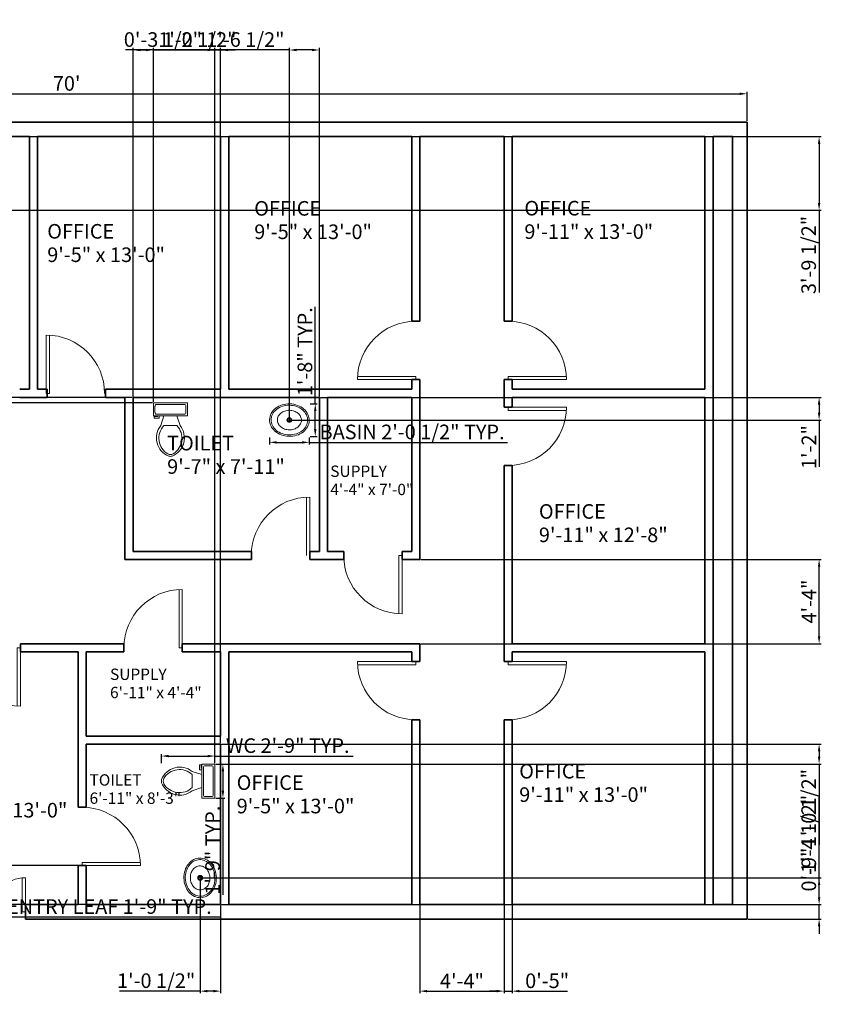
# Model space of a CAD drawing. Units: inches. Extents: x 2070 to 3026, y 1437 to 2044.
# Tile 2 of 2: x 2524 to 3026, y 1437 to 2044. Entities that reach past the tile are written whole.
import ezdxf

# ---------------------------------------------------------------- set-up
doc = ezdxf.new("R2010")
doc.units = ezdxf.units.IN
doc.layers.add('A-ANNO-DIMS', color=11, linetype='Continuous', lineweight=18, true_color=0xf27172)
for name, color, linetype, lineweight in [('A-AREA-IDEN', 7, 'Continuous', 18), ('A-DOOR', 4, 'Continuous', 18), ('A-FLOR-FIXT', 8, 'Continuous', 18), ('A-WALL', 7, 'Continuous', 35)]:
    doc.layers.add(name, color=color, linetype=linetype, lineweight=lineweight)
doc.styles.get("Standard").update_dxf_attribs({"font": 'arial.ttf'})
doc.dimstyles.new('ISO-25', dxfattribs={"dimtxt": 9, "dimasz": 4.5, "dimexe": 1.25, "dimexo": 0.625, "dimtad": 1, "dimdec": 0, "dimlunit": 3, "dimtxsty": 'Standard', "dimcen": 2.5, "dimadec": 0, "dimazin": 0, "dimtfac": 1, "dimtdec": 0, "dimtmove": 0, "dimatfit": 3, "dimfxl": 1, "dimarcsym": 0})

# ---------------------------------------------------------------- blocks, each defined once
blk = doc.blocks.new('Toilet - top')
for p, q in [((9.5, -6), (9.5, -2)), ((-10, -8.5), (-8, -8.5)), ((-10, -9.5), (-10, -8.5)), ((-7, -9.5), (-10, -9.5)), ((-8, -8.5), (-8, -8)), ((-7, -8), (-7, -9.5)), ((-4, -8), (-6, -14)), ((4, -8), (6, -14)), ((4, -14), (-4, -14))]:
    blk.add_line(p, q)
blk.add_lwpolyline([(10.5, -8), (10.5, 0), (-10.5, 0), (-10.5, -8)], close=True)
for points in [[(-9.5, -2), (-9.5, -6)], [(8.5, -1), (-8.5, -1)], [(-8.5, -7), (8.5, -7)]]:
    blk.add_lwpolyline(points)
for centre, radius, start, end in [((-8.62, -1.88), 0.884, 81.8699, 188.1301), ((-8.62, -6.12), 0.884, 171.8699, 278.1301), ((8.62, -1.88), 0.884, 351.8699, 98.1301), ((8.62, -6.12), 0.884, 261.8699, 8.1301), ((3.52, -21.58), 12.17, 141.46911, 247.97143), ((4.2, -21.82), 11.33, 136.36773, 238.94682), ((-3.52, -21.58), 12.17, 292.02843, 38.53071), ((-4.2, -21.82), 11.33, 301.05301, 43.63209), ((0, -27.88), 4, 245.73182, 294.26817), ((0, -29), 4, 254.86053, 285.13947)]:
    blk.add_arc(centre, radius, start, end)
blk = doc.blocks.new('Sink - Oval top')
for p, q in [((-1, 0), (1, 0)), ((0, 1), (0, -1))]:
    blk.add_line(p, q)
for points in [[(-12.23, 0.39, 0.117634), (-11.46, -3.36, 0.104469), (-8.88, -6.8, 0.090016), (-5.08, -9.07, 0.08192), (-0.32, -10.02, 0.08192), (4.49, -9.38, 0.090016), (8.42, -7.36, 0.104469), (11.22, -4.09, 0.117634), (12.23, -0.39, 0.117634), (11.46, 3.36, 0.104469), (8.88, 6.8, 0.090016), (5.08, 9.07, 0.08192), (0.32, 10.02, 0.08192), (-4.49, 9.38, 0.090016), (-8.42, 7.36, 0.104469), (-11.22, 4.09, 0.117634)], [(-11.29, 0.16, 0.118622), (-10.52, -3.25, 0.104678), (-8.07, -6.36, 0.089562), (-4.54, -8.37, 0.081185), (-0.13, -9.15, 0.081185), (4.3, -8.49, 0.089562), (7.89, -6.58, 0.104678), (10.42, -3.55, 0.118622), (11.29, -0.16, 0.118622), (10.52, 3.25, 0.104678), (8.07, 6.36, 0.089562), (4.54, 8.37, 0.081185), (0.13, 9.15, 0.081185), (-4.3, 8.49, 0.089562), (-7.89, 6.58, 0.104678), (-10.42, 3.55, 0.118622)], [(-7.42, 0.08, 0.118283), (-6.91, -2.17, 0.104607), (-5.29, -4.21, 0.089718), (-2.97, -5.53, 0.081436), (-0.07, -6.04, 0.081436), (2.84, -5.59, 0.089718), (5.2, -4.33, 0.104607), (6.86, -2.32, 0.118283), (7.42, -0.08, 0.118283), (6.91, 2.17, 0.104607), (5.29, 4.21, 0.089718), (2.97, 5.53, 0.081436), (0.07, 6.04, 0.081436), (-2.84, 5.59, 0.089718), (-5.2, 4.33, 0.104607), (-6.86, 2.32, 0.118283)]]:
    blk.add_lwpolyline(points, format="xyb", close=True)
for radius in [1.5, 1]:
    blk.add_circle((0, 0), radius)
blk = doc.blocks.new('*D3')
at = {"layer": 'A-ANNO-DIMS', "color": 0, "lineweight": -2, "transparency": 16777216}
for p, q in [((2133.31, 1981.8), (2133.31, 1999.85)), ((2973.31, 1981.8), (2973.31, 1999.85)), ((2137.81, 1998.6), (2968.81, 1998.6))]:
    blk.add_line(p, q, dxfattribs=at)
at = {"layer": 'A-ANNO-DIMS', "color": 0, "transparency": 16777216}
for points in [[(2137.81, 1999.35), (2137.81, 1997.85), (2133.31, 1998.6)], [(2968.81, 1999.35), (2968.81, 1997.85), (2973.31, 1998.6)]]:
    blk.add_solid(points, dxfattribs=at)
at = {"layer": 'Defpoints', "color": 0, "transparency": 16777216}
for p in [(2973.31, 1998.6), (2133.31, 1981.17), (2973.31, 1981.17)]:
    blk.add_point(p, dxfattribs=at)
at = {"layer": 'A-ANNO-DIMS', "color": 0, "transparency": 16777216, "insert": (2553.31, 2003.82), "char_height": 9, "attachment_point": 5}
blk.add_mtext("70'", dxfattribs=at)
blk = doc.blocks.new('DOOR-SWING-36IN')
for p, q in [((0, 2), (36, 2)), ((36, 0), (36, 2)), ((0, 0), (36, 0))]:
    blk.add_line(p, q)
blk.add_arc((36, 0), 36, 90, 180)
blk = doc.blocks.new('DOOR-ENTRY-LEAF-21IN')
for p, q in [((0, 21), (0, 0)), ((2, 21), (2, 0)), ((0, 0), (2, 0))]:
    blk.add_line(p, q)
blk.add_arc((0, 0), 21, 0, 90)
blk = doc.blocks.new('*D9')
at = {"layer": 'A-ANNO-DIMS', "color": 0, "lineweight": -2, "transparency": 16777216}
for p, q in [((2485.81, 1493.05), (2485.81, 1489.27)), ((2490.31, 1490.52), (2502.31, 1490.52)), ((2506.81, 1493.05), (2506.81, 1489.27)), ((2506.81, 1490.52), (2647.99, 1490.52))]:
    blk.add_line(p, q, dxfattribs=at)
at = {"layer": 'A-ANNO-DIMS', "color": 0, "transparency": 16777216}
for points in [[(2490.31, 1491.27), (2490.31, 1489.77), (2485.81, 1490.52)], [(2502.31, 1491.27), (2502.31, 1489.77), (2506.81, 1490.52)]]:
    blk.add_solid(points, dxfattribs=at)
at = {"layer": 'Defpoints', "color": 0, "transparency": 16777216}
for p in [(2485.81, 1493.67), (2506.81, 1493.67), (2506.81, 1490.52)]:
    blk.add_point(p, dxfattribs=at)
at = {"layer": 'A-ANNO-DIMS', "color": 0, "transparency": 16777216, "insert": (2579.65, 1495.74), "char_height": 9, "attachment_point": 5}
blk.add_mtext('ENTRY LEAF 1\'-9" TYP.', dxfattribs=at)
blk = doc.blocks.new('*D11')
at = {"layer": 'A-ANNO-DIMS', "color": 0, "lineweight": -2, "transparency": 16777216}
for p, q in [((2611.76, 1585.47), (2611.76, 1591.06)), ((2616.26, 1589.81), (2640.3, 1589.81)), ((2644.8, 1585.47), (2644.8, 1591.06)), ((2644.8, 1589.81), (2730.22, 1589.81))]:
    blk.add_line(p, q, dxfattribs=at)
at = {"layer": 'A-ANNO-DIMS', "color": 0, "transparency": 16777216}
for points in [[(2616.26, 1590.56), (2616.26, 1589.06), (2611.76, 1589.81)], [(2640.3, 1590.56), (2640.3, 1589.06), (2644.8, 1589.81)]]:
    blk.add_solid(points, dxfattribs=at)
at = {"layer": 'Defpoints', "color": 0, "transparency": 16777216}
for p in [(2644.8, 1589.81), (2611.76, 1584.85), (2644.8, 1584.85)]:
    blk.add_point(p, dxfattribs=at)
at = {"layer": 'A-ANNO-DIMS', "color": 0, "transparency": 16777216, "insert": (2689.76, 1595.08), "char_height": 9, "attachment_point": 5}
blk.add_mtext('WC 2\'-9" TYP.', dxfattribs=at)
blk = doc.blocks.new('*D12')
at = {"layer": 'A-ANNO-DIMS', "color": 0, "lineweight": -2, "transparency": 16777216}
for p, q in [((2645.43, 1584.85), (2651.01, 1584.85)), ((2649.76, 1580.35), (2649.76, 1568.35)), ((2645.43, 1563.85), (2651.01, 1563.85)), ((2649.76, 1563.85), (2649.76, 1504.09))]:
    blk.add_line(p, q, dxfattribs=at)
at = {"layer": 'A-ANNO-DIMS', "color": 0, "transparency": 16777216}
for points in [[(2649.01, 1580.35), (2650.51, 1580.35), (2649.76, 1584.85)], [(2649.01, 1568.35), (2650.51, 1568.35), (2649.76, 1563.85)]]:
    blk.add_solid(points, dxfattribs=at)
at = {"layer": 'Defpoints', "color": 0, "transparency": 16777216}
for p in [(2644.8, 1584.85), (2644.8, 1563.85), (2649.76, 1563.85)]:
    blk.add_point(p, dxfattribs=at)
at = {"layer": 'A-ANNO-DIMS', "color": 0, "transparency": 16777216, "insert": (2644.54, 1531.72), "char_height": 9, "attachment_point": 5, "rotation": 90}
blk.add_mtext('1\'-9" TYP.', dxfattribs=at)
blk = doc.blocks.new('*D13')
at = {"layer": 'A-ANNO-DIMS', "color": 0, "lineweight": -2, "transparency": 16777216}
for p, q in [((2678.51, 1786.49), (2678.51, 1782.18)), ((2683.01, 1783.43), (2698.56, 1783.43)), ((2703.06, 1786.49), (2703.06, 1782.18)), ((2703.06, 1783.43), (2825.46, 1783.43))]:
    blk.add_line(p, q, dxfattribs=at)
at = {"layer": 'A-ANNO-DIMS', "color": 0, "transparency": 16777216}
for points in [[(2683.01, 1784.18), (2683.01, 1782.68), (2678.51, 1783.43)], [(2698.56, 1784.18), (2698.56, 1782.68), (2703.06, 1783.43)]]:
    blk.add_solid(points, dxfattribs=at)
at = {"layer": 'Defpoints', "color": 0, "transparency": 16777216}
for p in [(2678.51, 1787.12), (2703.06, 1787.12), (2703.06, 1783.43)]:
    blk.add_point(p, dxfattribs=at)
at = {"layer": 'A-ANNO-DIMS', "color": 0, "transparency": 16777216, "insert": (2766.51, 1788.71), "char_height": 9, "attachment_point": 5}
blk.add_mtext('BASIN 2\'-0 1/2" TYP.', dxfattribs=at)
blk = doc.blocks.new('*D14')
at = {"layer": 'A-ANNO-DIMS', "color": 0, "lineweight": -2, "transparency": 16777216}
for p, q in [((2706.74, 1807.25), (2706.74, 1867.02)), ((2703.68, 1807.25), (2707.99, 1807.25)), ((2706.74, 1791.62), (2706.74, 1802.75)), ((2703.68, 1787.12), (2707.99, 1787.12))]:
    blk.add_line(p, q, dxfattribs=at)
at = {"layer": 'A-ANNO-DIMS', "color": 0, "transparency": 16777216}
for points in [[(2705.99, 1802.75), (2707.49, 1802.75), (2706.74, 1807.25)], [(2705.99, 1791.62), (2707.49, 1791.62), (2706.74, 1787.12)]]:
    blk.add_solid(points, dxfattribs=at)
at = {"layer": 'Defpoints', "color": 0, "transparency": 16777216}
for p in [(2703.06, 1807.25), (2706.74, 1807.25), (2703.06, 1787.12)]:
    blk.add_point(p, dxfattribs=at)
at = {"layer": 'A-ANNO-DIMS', "color": 0, "transparency": 16777216, "insert": (2701.52, 1839.38), "char_height": 9, "attachment_point": 5, "rotation": 90}
blk.add_mtext('1\'-8" TYP.', dxfattribs=at)
blk = doc.blocks.new('*D15')
at = {"layer": 'A-ANNO-DIMS', "color": 0, "lineweight": -2, "transparency": 16777216}
for p, q in [((2771.311043, 1497.547797), (2771.311043, 1443.472797)), ((2823.311043, 1497.547797), (2823.311043, 1443.472797)), ((2775.811043, 1444.722797), (2818.811043, 1444.722797))]:
    blk.add_line(p, q, dxfattribs=at)
at = {"layer": 'A-ANNO-DIMS', "color": 0, "transparency": 16777216}
for points in [[(2775.811043, 1445.472797), (2775.811043, 1443.972797), (2771.311043, 1444.722797)], [(2818.811043, 1445.472797), (2818.811043, 1443.972797), (2823.311043, 1444.722797)]]:
    blk.add_solid(points, dxfattribs=at)
at = {"layer": 'Defpoints', "color": 0, "transparency": 16777216}
for p in [(2771.311043, 1498.172797), (2823.311043, 1498.172797), (2823.311043, 1444.722797)]:
    blk.add_point(p, dxfattribs=at)
at = {"layer": 'A-ANNO-DIMS', "color": 0, "transparency": 16777216, "insert": (2797.311043, 1449.847797), "char_height": 9, "attachment_point": 5}
blk.add_mtext('4\'-4"', dxfattribs=at)
blk = doc.blocks.new('*D16')
at = {"layer": 'A-ANNO-DIMS', "color": 0, "lineweight": -2, "transparency": 16777216}
for p, q in [((2771.936043, 1711.172797), (3019.011043, 1711.172797)), ((3017.761043, 1663.672797), (3017.761043, 1706.672797)), ((2771.936043, 1659.172797), (3019.011043, 1659.172797))]:
    blk.add_line(p, q, dxfattribs=at)
at = {"layer": 'A-ANNO-DIMS', "color": 0, "transparency": 16777216}
for points in [[(3017.011043, 1706.672797), (3018.511043, 1706.672797), (3017.761043, 1711.172797)], [(3017.011043, 1663.672797), (3018.511043, 1663.672797), (3017.761043, 1659.172797)]]:
    blk.add_solid(points, dxfattribs=at)
at = {"layer": 'Defpoints', "color": 0, "transparency": 16777216}
for p in [(2771.311043, 1711.172797), (3017.761043, 1711.172797), (2771.311043, 1659.172797)]:
    blk.add_point(p, dxfattribs=at)
at = {"layer": 'A-ANNO-DIMS', "color": 0, "transparency": 16777216, "insert": (3012.636043, 1685.172797), "char_height": 9, "attachment_point": 5, "rotation": 90}
blk.add_mtext('4\'-4"', dxfattribs=at)
blk = doc.blocks.new('*D19')
at = {"layer": 'A-ANNO-DIMS', "color": 0, "lineweight": -2, "transparency": 16777216}
for p, q in [((2335.94, 1972.17), (3019.01, 1972.17)), ((3017.76, 1967.67), (3017.76, 1931.17)), ((2335.94, 1926.67), (3019.01, 1926.67)), ((3017.76, 1926.67), (3017.76, 1876.03))]:
    blk.add_line(p, q, dxfattribs=at)
at = {"layer": 'A-ANNO-DIMS', "color": 0, "transparency": 16777216}
for points in [[(3017.01, 1967.67), (3018.51, 1967.67), (3017.76, 1972.17)], [(3017.01, 1931.17), (3018.51, 1931.17), (3017.76, 1926.67)]]:
    blk.add_solid(points, dxfattribs=at)
at = {"layer": 'Defpoints', "color": 0, "transparency": 16777216}
for p in [(2335.31, 1972.17), (2335.31, 1926.67), (3017.76, 1926.67)]:
    blk.add_point(p, dxfattribs=at)
at = {"layer": 'A-ANNO-DIMS', "color": 0, "transparency": 16777216, "insert": (3012.48, 1899.1), "char_height": 9, "attachment_point": 5, "rotation": 90}
blk.add_mtext('3\'-9 1/2"', dxfattribs=at)
blk = doc.blocks.new('*D21')
at = {"layer": 'A-ANNO-DIMS', "color": 0, "lineweight": -2, "transparency": 16777216}
for p, q in [((2823.31, 1497.55), (2823.31, 1443.47)), ((2828.31, 1497.55), (2828.31, 1443.47)), ((2818.81, 1444.72), (2814.31, 1444.72)), ((2823.31, 1444.72), (2828.31, 1444.72)), ((2832.81, 1444.72), (2862.49, 1444.72))]:
    blk.add_line(p, q, dxfattribs=at)
at = {"layer": 'A-ANNO-DIMS', "color": 0, "transparency": 16777216}
for points in [[(2818.81, 1445.47), (2818.81, 1443.97), (2823.31, 1444.72)], [(2832.81, 1445.47), (2832.81, 1443.97), (2828.31, 1444.72)]]:
    blk.add_solid(points, dxfattribs=at)
at = {"layer": 'Defpoints', "color": 0, "transparency": 16777216}
for p in [(2823.31, 1498.17), (2828.31, 1498.17), (2828.31, 1444.72)]:
    blk.add_point(p, dxfattribs=at)
at = {"layer": 'A-ANNO-DIMS', "color": 0, "transparency": 16777216, "insert": (2849.9, 1449.94), "char_height": 9, "attachment_point": 5}
blk.add_mtext('0\'-5"', dxfattribs=at)
blk = doc.blocks.new('*D22')
at = {"layer": 'A-ANNO-DIMS', "color": 0, "lineweight": -2, "transparency": 16777216}
for p, q in [((3017.76, 1502.67), (3017.76, 1532.35)), ((2964.94, 1498.17), (3019.01, 1498.17)), ((3017.76, 1489.17), (3017.76, 1498.17)), ((2973.94, 1489.17), (3019.01, 1489.17)), ((3017.76, 1484.67), (3017.76, 1480.17))]:
    blk.add_line(p, q, dxfattribs=at)
at = {"layer": 'A-ANNO-DIMS', "color": 0, "transparency": 16777216}
for points in [[(3017.01, 1502.67), (3018.51, 1502.67), (3017.76, 1498.17)], [(3017.01, 1484.67), (3018.51, 1484.67), (3017.76, 1489.17)]]:
    blk.add_solid(points, dxfattribs=at)
at = {"layer": 'Defpoints', "color": 0, "transparency": 16777216}
for p in [(2964.31, 1498.17), (3017.76, 1498.17), (2973.31, 1489.17)]:
    blk.add_point(p, dxfattribs=at)
at = {"layer": 'A-ANNO-DIMS', "color": 0, "transparency": 16777216, "insert": (3012.54, 1519.76), "char_height": 9, "attachment_point": 5, "rotation": 90}
blk.add_mtext('0\'-9"', dxfattribs=at)
blk = doc.blocks.new('*D23')
at = {"layer": 'A-ANNO-DIMS', "color": 0, "lineweight": -2, "transparency": 16777216}
for p, q in [((2594.31, 1811.8), (2594.31, 2026.87)), ((2598.81, 2025.62), (2602.33, 2025.62)), ((2606.83, 1808.42), (2606.83, 2026.87)), ((2606.83, 2025.62), (2656.63, 2025.62))]:
    blk.add_line(p, q, dxfattribs=at)
at = {"layer": 'A-ANNO-DIMS', "color": 0, "transparency": 16777216}
for points in [[(2598.81, 2026.37), (2598.81, 2024.87), (2594.31, 2025.62)], [(2602.33, 2026.37), (2602.33, 2024.87), (2606.83, 2025.62)]]:
    blk.add_solid(points, dxfattribs=at)
at = {"layer": 'Defpoints', "color": 0, "transparency": 16777216}
for p in [(2606.83, 2025.62), (2594.31, 1811.17), (2606.83, 1807.8)]:
    blk.add_point(p, dxfattribs=at)
at = {"layer": 'A-ANNO-DIMS', "color": 0, "transparency": 16777216, "insert": (2633.98, 2030.9), "char_height": 9, "attachment_point": 5}
blk.add_mtext('1\'-0 1/2"', dxfattribs=at)
blk = doc.blocks.new('*D24')
at = {"layer": 'A-ANNO-DIMS', "color": 0, "lineweight": -2, "transparency": 16777216}
for p, q in [((2690.78, 2025.62), (2640.98, 2025.62)), ((2690.78, 1797.81), (2690.78, 2026.87)), ((2704.81, 2025.62), (2695.28, 2025.62)), ((2709.31, 1811.8), (2709.31, 2026.87))]:
    blk.add_line(p, q, dxfattribs=at)
at = {"layer": 'A-ANNO-DIMS', "color": 0, "transparency": 16777216}
for points in [[(2695.28, 2026.37), (2695.28, 2024.87), (2690.78, 2025.62)], [(2704.81, 2026.37), (2704.81, 2024.87), (2709.31, 2025.62)]]:
    blk.add_solid(points, dxfattribs=at)
at = {"layer": 'Defpoints', "color": 0, "transparency": 16777216}
for p in [(2690.78, 2025.62), (2709.31, 1811.17), (2690.78, 1797.19)]:
    blk.add_point(p, dxfattribs=at)
at = {"layer": 'A-ANNO-DIMS', "color": 0, "transparency": 16777216, "insert": (2663.63, 2030.9), "char_height": 9, "attachment_point": 5}
blk.add_mtext('1\'-6 1/2"', dxfattribs=at)
blk = doc.blocks.new('*D25')
at = {"layer": 'A-ANNO-DIMS', "color": 0, "lineweight": -2, "transparency": 16777216}
for p, q in [((2709.94, 1811.17), (3019.01, 1811.17)), ((3017.76, 1806.67), (3017.76, 1801.69)), ((2691.41, 1797.19), (3019.01, 1797.19)), ((3017.76, 1797.19), (3017.76, 1768.36))]:
    blk.add_line(p, q, dxfattribs=at)
at = {"layer": 'A-ANNO-DIMS', "color": 0, "transparency": 16777216}
for points in [[(3017.01, 1806.67), (3018.51, 1806.67), (3017.76, 1811.17)], [(3017.01, 1801.69), (3018.51, 1801.69), (3017.76, 1797.19)]]:
    blk.add_solid(points, dxfattribs=at)
at = {"layer": 'Defpoints', "color": 0, "transparency": 16777216}
for p in [(2709.31, 1811.17), (2690.78, 1797.19), (3017.76, 1797.19)]:
    blk.add_point(p, dxfattribs=at)
at = {"layer": 'A-ANNO-DIMS', "color": 0, "transparency": 16777216, "insert": (3012.62, 1780.52), "char_height": 9, "attachment_point": 5, "rotation": 90}
blk.add_mtext('1\'-2"', dxfattribs=at)
blk = doc.blocks.new('*D26')
at = {"layer": 'A-ANNO-DIMS', "color": 0, "lineweight": -2, "transparency": 16777216}
for p, q in [((2088.86, 1815.67), (2088.86, 1820.17)), ((2593.69, 1811.17), (2087.61, 1811.17)), ((2088.86, 1811.17), (2088.86, 1807.8)), ((2606.2, 1807.8), (2087.61, 1807.8)), ((2088.86, 1803.3), (2088.86, 1752.65))]:
    blk.add_line(p, q, dxfattribs=at)
at = {"layer": 'A-ANNO-DIMS', "color": 0, "transparency": 16777216}
for points in [[(2088.11, 1815.67), (2089.61, 1815.67), (2088.86, 1811.17)], [(2088.11, 1803.3), (2089.61, 1803.3), (2088.86, 1807.8)]]:
    blk.add_solid(points, dxfattribs=at)
at = {"layer": 'Defpoints', "color": 0, "transparency": 16777216}
for p in [(2594.31, 1811.17), (2088.86, 1807.8), (2606.83, 1807.8)]:
    blk.add_point(p, dxfattribs=at)
at = {"layer": 'A-ANNO-DIMS', "color": 0, "transparency": 16777216, "insert": (2083.58, 1775.72), "char_height": 9, "attachment_point": 5, "rotation": 90}
blk.add_mtext('0\'-3 1/2"', dxfattribs=at)
blk = doc.blocks.new('*D27')
at = {"layer": 'A-ANNO-DIMS', "color": 0, "lineweight": -2, "transparency": 16777216}
for p, q in [((2648.94, 1597.17), (3019.01, 1597.17)), ((3017.76, 1592.67), (3017.76, 1589.35)), ((2645.43, 1584.85), (3019.01, 1584.85)), ((3017.76, 1584.85), (3017.76, 1535.05))]:
    blk.add_line(p, q, dxfattribs=at)
at = {"layer": 'A-ANNO-DIMS', "color": 0, "transparency": 16777216}
for points in [[(3017.01, 1592.67), (3018.51, 1592.67), (3017.76, 1597.17)], [(3017.01, 1589.35), (3018.51, 1589.35), (3017.76, 1584.85)]]:
    blk.add_solid(points, dxfattribs=at)
at = {"layer": 'Defpoints', "color": 0, "transparency": 16777216}
for p in [(2648.31, 1597.17), (2644.8, 1584.85), (3017.76, 1584.85)]:
    blk.add_point(p, dxfattribs=at)
at = {"layer": 'A-ANNO-DIMS', "color": 0, "transparency": 16777216, "insert": (3012.48, 1557.7), "char_height": 9, "attachment_point": 5, "rotation": 90}
blk.add_mtext('1\'-0 1/2"', dxfattribs=at)
blk = doc.blocks.new('*D28')
at = {"layer": 'A-ANNO-DIMS', "color": 0, "lineweight": -2, "transparency": 16777216}
for p, q in [((3017.76, 1514.62), (3017.76, 1564.41)), ((2636.32, 1514.62), (3019.01, 1514.62)), ((3017.76, 1502.67), (3017.76, 1510.12)), ((2648.94, 1498.17), (3019.01, 1498.17))]:
    blk.add_line(p, q, dxfattribs=at)
at = {"layer": 'A-ANNO-DIMS', "color": 0, "transparency": 16777216}
for points in [[(3017.01, 1510.12), (3018.51, 1510.12), (3017.76, 1514.62)], [(3017.01, 1502.67), (3018.51, 1502.67), (3017.76, 1498.17)]]:
    blk.add_solid(points, dxfattribs=at)
at = {"layer": 'Defpoints', "color": 0, "transparency": 16777216}
for p in [(2635.69, 1514.62), (3017.76, 1514.62), (2648.31, 1498.17)]:
    blk.add_point(p, dxfattribs=at)
at = {"layer": 'A-ANNO-DIMS', "color": 0, "transparency": 16777216, "insert": (3012.48, 1541.76), "char_height": 9, "attachment_point": 5, "rotation": 90}
blk.add_mtext('1\'-4 1/2"', dxfattribs=at)
blk = doc.blocks.new('*D29')
at = {"layer": 'A-ANNO-DIMS', "color": 0, "lineweight": -2, "transparency": 16777216}
for p, q in [((2635.69, 1513.99), (2635.69, 1443.47)), ((2648.31, 1497.55), (2648.31, 1443.47)), ((2635.69, 1444.72), (2585.9, 1444.72)), ((2643.81, 1444.72), (2640.19, 1444.72))]:
    blk.add_line(p, q, dxfattribs=at)
at = {"layer": 'A-ANNO-DIMS', "color": 0, "transparency": 16777216}
for points in [[(2640.19, 1445.47), (2640.19, 1443.97), (2635.69, 1444.72)], [(2643.81, 1445.47), (2643.81, 1443.97), (2648.31, 1444.72)]]:
    blk.add_solid(points, dxfattribs=at)
at = {"layer": 'Defpoints', "color": 0, "transparency": 16777216}
for p in [(2635.69, 1514.62), (2648.31, 1498.17), (2635.69, 1444.72)]:
    blk.add_point(p, dxfattribs=at)
at = {"layer": 'A-ANNO-DIMS', "color": 0, "transparency": 16777216, "insert": (2608.55, 1450), "char_height": 9, "attachment_point": 5}
blk.add_mtext('1\'-0 1/2"', dxfattribs=at)
blk = doc.blocks.new('*D30')
at = {"layer": 'A-ANNO-DIMS', "color": 0, "lineweight": -2, "transparency": 16777216}
for p, q in [((2640.3, 2025.62), (2589.66, 2025.62)), ((2644.8, 1585.47), (2644.8, 2026.87)), ((2648.31, 2025.62), (2644.8, 2025.62)), ((2648.31, 1597.8), (2648.31, 2026.87)), ((2652.81, 2025.62), (2657.31, 2025.62))]:
    blk.add_line(p, q, dxfattribs=at)
at = {"layer": 'A-ANNO-DIMS', "color": 0, "transparency": 16777216}
for points in [[(2640.3, 2026.37), (2640.3, 2024.87), (2644.8, 2025.62)], [(2652.81, 2026.37), (2652.81, 2024.87), (2648.31, 2025.62)]]:
    blk.add_solid(points, dxfattribs=at)
at = {"layer": 'Defpoints', "color": 0, "transparency": 16777216}
for p in [(2644.8, 2025.62), (2648.31, 1597.17), (2644.8, 1584.85)]:
    blk.add_point(p, dxfattribs=at)
at = {"layer": 'A-ANNO-DIMS', "color": 0, "transparency": 16777216, "insert": (2612.73, 2030.9), "char_height": 9, "attachment_point": 5}
blk.add_mtext('0\'-3 1/2"', dxfattribs=at)
blk = doc.blocks.new('*D31')
at = {"layer": 'A-ANNO-DIMS', "color": 0, "lineweight": -2, "transparency": 16777216}
for p, q in [((2564.69, 1522.17), (2087.61, 1522.17)), ((2088.86, 1517.67), (2088.86, 1502.67)), ((2564.69, 1498.17), (2087.61, 1498.17)), ((2088.86, 1498.17), (2088.86, 1468.35))]:
    blk.add_line(p, q, dxfattribs=at)
at = {"layer": 'A-ANNO-DIMS', "color": 0, "transparency": 16777216}
for points in [[(2088.11, 1517.67), (2089.61, 1517.67), (2088.86, 1522.17)], [(2088.11, 1502.67), (2089.61, 1502.67), (2088.86, 1498.17)]]:
    blk.add_solid(points, dxfattribs=at)
at = {"layer": 'Defpoints', "color": 0, "transparency": 16777216}
for p in [(2565.31, 1522.17), (2088.86, 1498.17), (2565.31, 1498.17)]:
    blk.add_point(p, dxfattribs=at)
at = {"layer": 'A-ANNO-DIMS', "color": 0, "transparency": 16777216, "insert": (2083.64, 1481.01), "char_height": 9, "attachment_point": 5, "rotation": 90}
blk.add_mtext('2\'-0"', dxfattribs=at)

msp = doc.modelspace()

# ---------------------------------------------------------------- linework, layer by layer
at = {"layer": 'A-DOOR'}
for p, q in [((2701.31, 1749.67), (2701.31, 1713.67)), ((2703.31, 1749.67), (2703.31, 1713.67))]:
    msp.add_line(p, q, dxfattribs=at)
msp.add_arc((2703.31, 1713.67), 36, 90, 180, dxfattribs=at)
at = {"layer": 'A-WALL'}
for p, q in [((2133.31, 1981.17), (2973.31, 1981.17)), ((2973.31, 1981.17), (2973.31, 1489.17)), ((2417.31, 1972.17), (2530.31, 1972.17)), ((2530.31, 1816.17), (2530.31, 1972.17)), ((2535.31, 1816.17), (2535.31, 1972.17)), ((2535.31, 1972.17), (2648.31, 1972.17)), ((2648.31, 1816.17), (2648.31, 1972.17)), ((2648.31, 1816.17), (2648.31, 1972.17)), ((2653.31, 1816.17), (2653.31, 1972.17)), ((2653.31, 1816.17), (2653.31, 1972.17)), ((2653.31, 1972.17), (2766.31, 1972.17)), ((2766.31, 1858.17), (2766.31, 1972.17)), ((2771.31, 1858.17), (2771.31, 1972.17)), ((2771.31, 1972.17), (2823.31, 1972.17)), ((2823.31, 1858.17), (2823.31, 1972.17)), ((2828.31, 1858.17), (2828.31, 1972.17)), ((2828.31, 1972.17), (2947.31, 1972.17)), ((2947.31, 1972.17), (2947.31, 1816.17)), ((2952.31, 1972.17), (2952.31, 1498.17)), ((2952.31, 1972.17), (2964.31, 1972.17)), ((2964.31, 1972.17), (2964.31, 1498.17)), ((2766.31, 1858.17), (2771.31, 1858.17)), ((2823.31, 1858.17), (2828.31, 1858.17)), ((2766.31, 1822.17), (2771.31, 1822.17)), ((2766.31, 1816.17), (2766.31, 1822.17)), ((2771.31, 1711.17), (2771.31, 1822.17)), ((2823.31, 1822.17), (2828.31, 1822.17)), ((2823.31, 1805.17), (2823.31, 1822.17)), ((2828.31, 1816.17), (2828.31, 1822.17)), ((2524.31, 1816.17), (2530.31, 1816.17)), ((2524.31, 1811.17), (2541.31, 1811.17)), ((2535.31, 1816.17), (2541.31, 1816.17)), ((2541.31, 1811.17), (2541.31, 1816.17)), ((2577.31, 1811.17), (2577.31, 1816.17)), ((2577.31, 1816.17), (2648.31, 1816.17)), ((2577.31, 1811.17), (2589.31, 1811.17)), ((2589.31, 1711.17), (2589.31, 1811.17)), ((2594.31, 1716.17), (2594.31, 1811.17)), ((2594.31, 1811.17), (2709.31, 1811.17)), ((2653.31, 1816.17), (2766.31, 1816.17)), ((2709.31, 1716.17), (2709.31, 1811.17)), ((2714.31, 1716.17), (2714.31, 1811.17)), ((2714.31, 1811.17), (2766.31, 1811.17)), ((2766.31, 1716.17), (2766.31, 1811.17)), ((2828.31, 1816.17), (2947.31, 1816.17)), ((2828.31, 1811.17), (2947.31, 1811.17)), ((2828.31, 1805.17), (2828.31, 1811.17)), ((2947.31, 1811.17), (2947.31, 1659.17)), ((2823.31, 1805.17), (2828.31, 1805.17)), ((2823.31, 1648.17), (2823.31, 1769.17)), ((2823.31, 1769.17), (2828.31, 1769.17)), ((2828.31, 1659.17), (2828.31, 1769.17)), ((2594.31, 1716.17), (2667.31, 1716.17)), ((2667.31, 1711.17), (2667.31, 1716.17)), ((2703.31, 1711.17), (2703.31, 1716.17)), ((2703.31, 1716.17), (2709.31, 1716.17)), ((2714.31, 1716.17), (2724.31, 1716.17)), ((2724.31, 1711.17), (2724.31, 1716.17)), ((2760.31, 1716.17), (2766.31, 1716.17)), ((2760.31, 1711.17), (2760.31, 1716.17)), ((2589.31, 1711.17), (2667.31, 1711.17)), ((2703.31, 1711.17), (2724.31, 1711.17)), ((2760.31, 1711.17), (2771.31, 1711.17)), ((2524.81, 1654.17), (2524.81, 1659.17)), ((2588.69, 1659.17), (2524.81, 1659.17)), ((2588.69, 1654.17), (2588.69, 1659.17)), ((2771.31, 1659.17), (2624.69, 1659.17)), ((2624.69, 1654.17), (2624.69, 1659.17)), ((2771.31, 1648.17), (2771.31, 1659.17)), ((2947.31, 1659.17), (2828.31, 1659.17)), ((2524.81, 1654.17), (2560.31, 1654.17)), ((2560.31, 1654.17), (2524.81, 1654.17)), ((2560.31, 1558.17), (2560.31, 1654.17)), ((2565.31, 1654.17), (2588.69, 1654.17)), ((2588.69, 1654.17), (2565.31, 1654.17)), ((2565.31, 1602.17), (2565.31, 1654.17)), ((2624.69, 1654.17), (2648.06, 1654.17)), ((2648.31, 1654.17), (2624.69, 1654.17)), ((2648.31, 1602.17), (2648.31, 1654.17)), ((2653.31, 1498.17), (2653.31, 1654.17)), ((2766.31, 1654.17), (2653.31, 1654.17)), ((2766.31, 1648.17), (2766.31, 1654.17)), ((2947.31, 1654.17), (2828.31, 1654.17)), ((2828.31, 1648.17), (2828.31, 1654.17)), ((2947.31, 1654.17), (2947.31, 1498.17)), ((2771.31, 1648.17), (2766.31, 1648.17)), ((2828.31, 1648.17), (2823.31, 1648.17)), ((2766.31, 1498.17), (2766.31, 1612.17)), ((2771.31, 1612.17), (2766.31, 1612.17)), ((2771.31, 1498.17), (2771.31, 1612.17)), ((2823.31, 1498.17), (2823.31, 1612.17)), ((2828.31, 1612.17), (2823.31, 1612.17)), ((2828.31, 1498.17), (2828.31, 1612.17)), ((2648.31, 1602.17), (2565.31, 1602.17)), ((2648.31, 1597.17), (2565.31, 1597.17)), ((2565.31, 1558.17), (2565.31, 1597.17)), ((2648.31, 1498.17), (2648.31, 1597.17)), ((2565.31, 1558.17), (2560.31, 1558.17)), ((2560.31, 1498.17), (2560.31, 1522.17)), ((2565.31, 1522.17), (2560.31, 1522.17)), ((2565.31, 1498.17), (2565.31, 1522.17)), ((2560.31, 1498.17), (2527.81, 1498.17)), ((2527.81, 1498.17), (2527.81, 1489.17)), ((2560.31, 1498.17), (2527.81, 1498.17)), ((2648.31, 1498.17), (2565.31, 1498.17)), ((2766.31, 1498.17), (2653.31, 1498.17)), ((2823.31, 1498.17), (2771.31, 1498.17)), ((2947.31, 1498.17), (2828.31, 1498.17)), ((2964.31, 1498.17), (2952.31, 1498.17)), ((2973.31, 1489.17), (2527.81, 1489.17))]:
    msp.add_line(p, q, dxfattribs=at)

# ---------------------------------------------------------------- block references
at = {"layer": 'A-DOOR'}
msp.add_blockref('DOOR-SWING-36IN', (2732.81, 1822.17), dxfattribs=at)
at = {"layer": 'A-DOOR', "extrusion": (0, 0, -1), "zscale": -1}
for name, p in [('DOOR-SWING-36IN', (-2861.81, 1822.17)), ('DOOR-SWING-36IN', (-2598.81, 1522.17)), ('DOOR-ENTRY-LEAF-21IN', (-2527.81, 1493.67))]:
    msp.add_blockref(name, p, dxfattribs=at)
at = {"layer": 'A-DOOR'}
for p, rotation in [((2540.73, 1849.67), 270.0000000000001), ((2861.81, 1805.17), 180), ((2760.31, 1677.67), 89.99999999999984), ((2524.81, 1620.67), 89.99999999999994), ((2861.81, 1648.17), 180)]:
    msp.add_blockref('DOOR-SWING-36IN', p, dxfattribs=dict(at, rotation=rotation))
at = {"layer": 'A-DOOR', "extrusion": (0, 0, -1), "zscale": -1}
for p, rotation in [((-2624.69, 1692.67), 269.9999999999992), ((-2732.81, 1648.17), 180)]:
    msp.add_blockref('DOOR-SWING-36IN', p, dxfattribs=dict(at, rotation=rotation))
at = {"layer": 'A-FLOR-FIXT'}
for name, p in [('Toilet - top', (2617.33, 1807.8)), ('Sink - Oval top', (2690.78, 1797.19))]:
    msp.add_blockref(name, p, dxfattribs=at)
for name, p, rotation in [('Toilet - top', (2644.8, 1574.35), 270), ('Sink - Oval top', (2635.69, 1514.62), 93.00912233990628)]:
    msp.add_blockref(name, p, dxfattribs=dict(at, rotation=rotation))

# ---------------------------------------------------------------- texts
at = {"layer": 'A-AREA-IDEN'}
for s, height, p in [('OFFICE', 9, (2835.84, 1923.49)), ('OFFICE', 9, (2669.08, 1923.38)), ('OFFICE', 9, (2541.32, 1909.2)), ('9\'-5" x 13\'-0"', 9, (2669.08, 1908.92)), ('9\'-11" x 13\'-0"', 9, (2835.84, 1909.03)), ('9\'-5" x 13\'-0"', 9, (2541.32, 1894.75)), ('TOILET', 9, (2615.32, 1778.47)), ('9\'-7" x 7\'-11"', 9, (2615.32, 1764.01)), ('SUPPLY', 7, (2716.03, 1762.11)), ('4\'-4" x 7\'-0"', 7, (2716.03, 1750.86)), ('OFFICE', 9, (2844.8, 1736.3)), ('9\'-11" x 12\'-8"', 9, (2844.8, 1721.84)), ('SUPPLY', 7, (2580.08, 1636.78)), ('6\'-11" x 4\'-4"', 7, (2580.08, 1625.53)), ('OFFICE', 9, (2832.65, 1575.97)), ('TOILET  ', 7, (2567.43, 1571.56)), ('OFFICE', 9, (2658.24, 1568.92)), ('9\'-11" x 13\'-0"', 9, (2832.65, 1561.51)), ('6\'-11" x 8\'-3"', 7, (2567.43, 1560.32)), ('9\'-5" x 13\'-0"', 9, (2658.24, 1554.46)), ('8\'-11" x 13\'-0"', 9, (2474.24, 1551.9))]:
    msp.add_text(s, height=height, dxfattribs=at).set_placement(p)

# ---------------------------------------------------------------- dimensions: what is measured, and where the dimension line sits
at = {"layer": 'A-ANNO-DIMS'}
for base, p1, p2, override, picture, middle in [((2644.8, 2025.62), (2648.31, 1597.17), (2644.8, 1584.85), {"dimdec": 1, "dimlfac": 1, "dimrnd": 0, "dimzin": 1, "dimdsep": 46, "dimlunit": 4, "dimfrac": 2}, '*D30', (2612.73, 2030.9)), ((2606.83, 2025.62), (2594.31, 1811.17), (2606.83, 1807.8), {"dimdec": 1, "dimlfac": 1, "dimrnd": 0, "dimzin": 1, "dimdsep": 46, "dimlunit": 4, "dimfrac": 2}, '*D23', (2633.98, 2030.9)), ((2690.78, 2025.62), (2709.31, 1811.17), (2690.78, 1797.19), {"dimdec": 1, "dimlfac": 1, "dimrnd": 0, "dimzin": 1, "dimdsep": 46, "dimlunit": 4, "dimfrac": 2}, '*D24', (2663.63, 2030.9)), ((2973.31, 1998.6), (2133.31, 1981.17), (2973.31, 1981.17), {"dimclrd": 0, "dimclre": 0, "dimclrt": 0}, '*D3', (2553.31, 2003.82)), ((2635.69, 1444.72), (2648.31, 1498.17), (2635.69, 1514.62), {"dimdec": 1, "dimlfac": 1, "dimrnd": 0, "dimzin": 1, "dimdsep": 46, "dimlunit": 4, "dimfrac": 2}, '*D29', (2608.55, 1450)), ((2823.31, 1444.72), (2771.31, 1498.17), (2823.31, 1498.17), {"dimdec": 1, "dimlfac": 1, "dimrnd": 0, "dimzin": 1, "dimdsep": 46, "dimlunit": 4, "dimfrac": 2}, '*D15', (2797.31, 1449.85)), ((2828.31, 1444.72), (2823.31, 1498.17), (2828.31, 1498.17), {"dimdec": 1, "dimlfac": 1, "dimrnd": 0, "dimzin": 1, "dimdsep": 46, "dimlunit": 4, "dimfrac": 2}, '*D21', (2849.9, 1449.94))]:
    dim = msp.add_linear_dim(base=base, p1=p1, p2=p2, dimstyle='ISO-25', override=override, dxfattribs=at)
    dim.commit()
    dim.dimension.update_dxf_attribs({"geometry": picture, "text_midpoint": middle})
for base, p1, p2, picture, middle in [((3017.76, 1926.67), (2335.31, 1972.17), (2335.31, 1926.67), '*D19', (3012.48, 1899.1)), ((2088.86, 1807.8), (2594.31, 1811.17), (2606.83, 1807.8), '*D26', (2083.58, 1775.72)), ((3017.76, 1797.19), (2709.31, 1811.17), (2690.78, 1797.19), '*D25', (3012.62, 1780.52)), ((3017.76, 1711.17), (2771.31, 1659.17), (2771.31, 1711.17), '*D16', (3012.64, 1685.17)), ((3017.76, 1584.85), (2648.31, 1597.17), (2644.8, 1584.85), '*D27', (3012.48, 1557.7)), ((3017.761, 1514.6157), (2648.311, 1498.1728), (2635.6947, 1514.6157), '*D28', (3012.4826, 1541.7649)), ((3017.76, 1498.17), (2973.31, 1489.17), (2964.31, 1498.17), '*D22', (3012.54, 1519.76)), ((2088.86, 1498.17), (2565.31, 1522.17), (2565.31, 1498.17), '*D31', (2083.64, 1481.01))]:
    dim = msp.add_linear_dim(base=base, p1=p1, p2=p2, angle=90, dimstyle='ISO-25', override={"dimdec": 1, "dimlfac": 1, "dimrnd": 0, "dimzin": 1, "dimdsep": 46, "dimlunit": 4, "dimfrac": 2}, dxfattribs=at)
    dim.commit()
    dim.dimension.update_dxf_attribs({"geometry": picture, "text_midpoint": middle})
for base, p1, p2, angle, picture, middle in [((2706.74, 1807.25), (2703.06, 1787.12), (2703.06, 1807.25), 90, '*D14', (2701.52, 1839.38)), ((2649.76, 1563.85), (2644.8, 1584.85), (2644.8, 1563.85), 270, '*D12', (2644.54, 1531.72))]:
    dim = msp.add_linear_dim(base=base, p1=p1, p2=p2, angle=angle, text='<> TYP.', dimstyle='ISO-25', override={"dimdec": 1, "dimlfac": 1, "dimrnd": 0, "dimzin": 1, "dimdsep": 46, "dimlunit": 4, "dimfrac": 2}, dxfattribs=at)
    dim.commit()
    dim.dimension.update_dxf_attribs({"geometry": picture, "text_midpoint": middle})
for base, p1, p2, text, picture, middle in [((2703.0585, 1783.4345), (2678.5076, 1787.1172), (2703.0585, 1787.1172), 'BASIN <> TYP.', '*D13', (2766.5116, 1788.713)), ((2644.8, 1589.81), (2611.76, 1584.85), (2644.8, 1584.85), 'WC <> TYP.', '*D11', (2689.76, 1595.08)), ((2506.81, 1490.52), (2485.81, 1493.67), (2506.81, 1493.67), 'ENTRY LEAF <> TYP.', '*D9', (2579.65, 1495.74))]:
    dim = msp.add_linear_dim(base=base, p1=p1, p2=p2, text=text, dimstyle='ISO-25', override={"dimdec": 1, "dimlfac": 1, "dimrnd": 0, "dimzin": 1, "dimdsep": 46, "dimlunit": 4, "dimfrac": 2}, dxfattribs=at)
    dim.commit()
    dim.dimension.update_dxf_attribs({"geometry": picture, "text_midpoint": middle})

doc.saveas('drawing.dxf')
